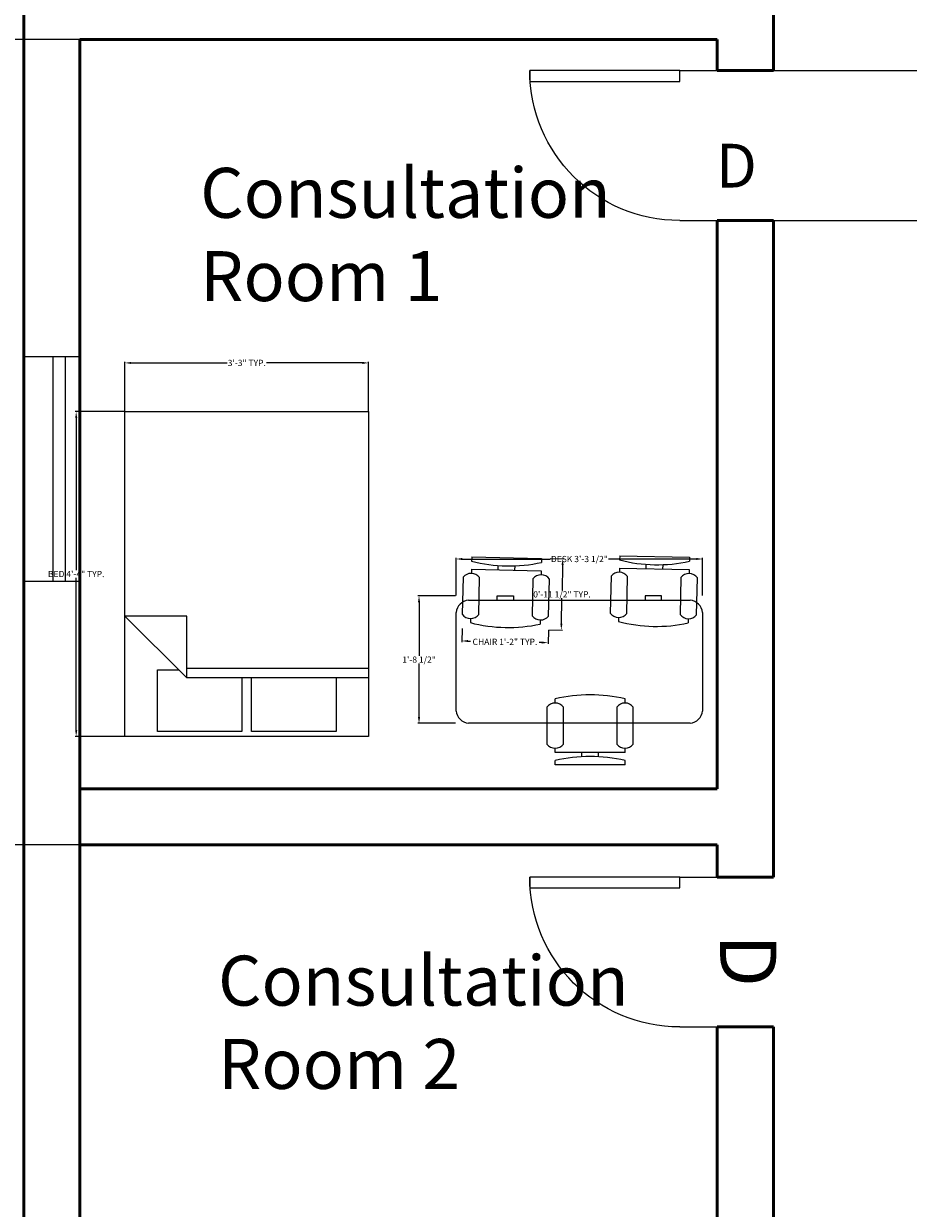
# Model space of a CAD drawing. Units: inches. Extents: x -364 to 705, y -52 to 1250.
# Tile 22 of 34: x 29 to 170, y 648 to 838. Entities that reach past the tile are written whole.
import ezdxf

# ---------------------------------------------------------------- set-up
doc = ezdxf.new("R2010")
doc.units = ezdxf.units.IN
doc.header["$MEASUREMENT"] = 0
for name, color, linetype, lineweight in [('A-ANNO-DIMS', 4, 'Continuous', 18), ('A-ANNO-IDEN', 1, 'Continuous', 18), ('A-AREA-IDEN', 3, 'Continuous', 18), ('A-DOOR', 1, 'Continuous', 25), ('A-FURN', 8, 'Continuous', 18), ('A-GLAZ', 4, 'Continuous', 25), ('A-WALL', 41, 'Continuous', 50)]:
    doc.layers.add(name, color=color, linetype=linetype, lineweight=lineweight)
doc.styles.get("Standard").update_dxf_attribs({"font": 'arial.ttf'})
doc.dimstyles.get("Standard").update_dxf_attribs({"dimtxt": 1, "dimasz": 1, "dimexe": 0.18, "dimexo": 0.0625, "dimgap": 0.09, "dimtad": 0, "dimtih": 1, "dimtoh": 1, "dimdec": 0, "dimzin": 0, "dimdsep": 46, "dimlunit": 3, "dimtxsty": 'Standard', "dimcen": 0.09, "dimadec": 0, "dimazin": 0, "dimtfac": 1, "dimtdec": 0, "dimtofl": 0, "dimtmove": 0, "dimatfit": 3, "dimfxl": 1, "dimtolj": 1, "dimtzin": 0, "dimarcsym": 0})

# ---------------------------------------------------------------- blocks, each defined once
blk = doc.blocks.new('Chair - Desk')
for p, q in [((-8.5, 0), (-8.5, -1)), ((-8.5, 0), (8.5, 0)), ((8.5, 0), (8.5, -1)), ((-2, -3), (-2, -1.9355)), ((2, -1.9576), (2, -3)), ((-10.5, -5), (-10.5, -14)), ((-8.5, -3), (-8.5, -4)), ((-8.5, -3), (8.5, -3)), ((-6.5, -14), (-6.5, -5)), ((6.5, -5), (6.5, -14)), ((8.5, -3), (8.5, -4)), ((10.5, -14), (10.5, -5)), ((-8.5, -15), (-8.5, -16)), ((8.5, -15), (8.5, -16))]:
    blk.add_line(p, q)
for centre, radius, start, end in [((0, 34.625), 36.625, 256.5803, 283.4197), ((-8.5, -6.5), 2.5, 36.8699, 143.1301), ((8.5, -6.5), 2.5, 36.8699, 143.1301), ((-8.5, -12.5), 2.5, 216.8699, 323.1301), ((8.5, -12.5), 2.5, 216.8699, 323.1301), ((0, 19.625), 36.625, 256.5803, 283.4197)]:
    blk.add_arc(centre, radius, start, end)
blk = doc.blocks.new('Desk - 30 x 60 in.')
for p, q in [((-26.999995, 0), (26.999995, 0)), ((-29.999995, -27), (-29.999995, -3)), ((29.999995, -3), (29.999995, -27)), ((26.999995, -30), (-26.999995, -30)), ((-20.000005, -30), (-20.000005, -31)), ((-20.000005, -31), (-16.000005, -31)), ((-16.000005, -31), (-16.000005, -30)), ((15.999995, -31), (15.999995, -30)), ((19.999995, -31), (15.999995, -31)), ((19.999995, -30), (19.999995, -31))]:
    blk.add_line(p, q)
for centre, start, end in [((-26.499995, -3.5), 98.1301, 171.8699), ((26.499995, -3.5), 8.130102, 81.8699), ((-26.499995, -26.5), 188.1301, 261.8699), ((26.499995, -26.5), 278.1301, 351.8699)]:
    blk.add_arc(centre, 3.535534, start, end)
blk = doc.blocks.new('Bed - Queen')
for p, q in [((0, -80.00003), (0, 0)), ((0, 0), (59.99999, 0)), ((59.99999, 0), (59.99999, -80.00003)), ((7.99999, -1.2), (28.79998, -1.2)), ((7.99999, -14.4), (7.99999, -1.2)), ((28.79998, -1.2), (28.79998, -14.4)), ((31.19999, -1.2), (51.99999, -1.2)), ((31.19999, -14.4), (31.19999, -1.2)), ((51.99999, -1.2), (51.99999, -16.4)), ((0, -14.4), (44.8, -14.4)), ((59.99999, -29.6), (44.8, -14.4)), ((44.8, -14.4), (44.8, -29.6)), ((44.8, -16.8), (0, -16.8)), ((51.99999, -16.4), (46.79936, -16.4)), ((44.8, -29.6), (59.99999, -29.6)), ((59.99999, -80.00003), (0, -80.00003))]:
    blk.add_line(p, q)
blk = doc.blocks.new('*U16')
for p, q in [((-24, 0), (-24, 6)), ((0, 0), (0, 6))]:
    blk.add_line(p, q)
blk.add_lwpolyline([(0, 0), (0, -24), (-1.75, -24), (-1.75, 0)], close=True)
blk.add_arc((0, 0), 24, 180, 270)
blk = doc.blocks.new('*D19')
at = {"layer": 'A-ANNO-DIMS', "color": 0, "lineweight": -2, "transparency": 16777216}
for p, q in [((28.52, 986.11), (-248.33, 986.11)), ((-248.15, 985.11), (-248.15, 574.22)), ((-248.15, 149.87), (-248.15, 560.77)), ((28.52, 148.87), (-248.33, 148.87))]:
    blk.add_line(p, q, dxfattribs=at)
at = {"layer": 'A-ANNO-DIMS', "color": 0, "transparency": 16777216}
for points in [[(-248.32, 985.11), (-247.99, 985.11), (-248.15, 986.11)], [(-248.32, 149.87), (-247.99, 149.87), (-248.15, 148.87)]]:
    blk.add_solid(points, dxfattribs=at)
at = {"layer": 'Defpoints', "color": 0, "transparency": 16777216}
for p in [(28.58, 986.11), (-248.15, 148.87), (28.58, 148.87)]:
    blk.add_point(p, dxfattribs=at)
at = {"layer": 'A-ANNO-DIMS', "color": 0, "transparency": 16777216, "insert": (-248.15, 567.49), "char_height": 1, "attachment_point": 5}
blk.add_mtext('\\A1;{\\H13x;69\'-9"}', dxfattribs=at)
blk = doc.blocks.new('*D20')
at = {"layer": 'A-ANNO-DIMS', "color": 0, "lineweight": -2, "transparency": 16777216}
for p, q in [((28.52, 986.11), (-188.21, 986.11)), ((-188.03, 985.11), (-188.03, 917.23)), ((-188.03, 836.11), (-188.03, 904)), ((37.52, 835.11), (-188.21, 835.11))]:
    blk.add_line(p, q, dxfattribs=at)
at = {"layer": 'A-ANNO-DIMS', "color": 0, "transparency": 16777216}
for points in [[(-188.19, 985.11), (-187.86, 985.11), (-188.03, 986.11)], [(-188.19, 836.11), (-187.86, 836.11), (-188.03, 835.11)]]:
    blk.add_solid(points, dxfattribs=at)
at = {"layer": 'Defpoints', "color": 0, "transparency": 16777216}
for p in [(28.58, 986.11), (-188.03, 835.11), (37.58, 835.11)]:
    blk.add_point(p, dxfattribs=at)
at = {"layer": 'A-ANNO-DIMS', "color": 0, "transparency": 16777216, "insert": (-188.03, 910.61), "char_height": 1, "attachment_point": 5}
blk.add_mtext('\\A1;{\\H13x;12\'-7"}', dxfattribs=at)
blk = doc.blocks.new('*D21')
at = {"layer": 'A-ANNO-DIMS', "color": 0, "lineweight": -2, "transparency": 16777216}
for p, q in [((37.52, 835.11), (-188.94, 835.11)), ((-188.76, 834.11), (-188.76, 777.34)), ((-188.76, 707.11), (-188.76, 763.89)), ((37.52, 706.11), (-188.94, 706.11))]:
    blk.add_line(p, q, dxfattribs=at)
at = {"layer": 'A-ANNO-DIMS', "color": 0, "transparency": 16777216}
for points in [[(-188.93, 834.11), (-188.59, 834.11), (-188.76, 835.11)], [(-188.93, 707.11), (-188.59, 707.11), (-188.76, 706.11)]]:
    blk.add_solid(points, dxfattribs=at)
at = {"layer": 'Defpoints', "color": 0, "transparency": 16777216}
for p in [(37.58, 835.11), (-188.76, 706.11), (37.58, 706.11)]:
    blk.add_point(p, dxfattribs=at)
at = {"layer": 'A-ANNO-DIMS', "color": 0, "transparency": 16777216, "insert": (-188.76, 770.61), "char_height": 1, "attachment_point": 5}
blk.add_mtext('\\A1;{\\H13x;10\'-9"}', dxfattribs=at)
blk = doc.blocks.new('*D31')
at = {"layer": 'A-ANNO-DIMS', "color": 0, "lineweight": -2, "transparency": 16777216}
for p, q in [((37.52, 706.11), (-205.07, 706.11)), ((-204.89, 705.11), (-204.89, 648.34)), ((-204.89, 578.11), (-204.89, 634.89)), ((37.52, 577.11), (-205.07, 577.11))]:
    blk.add_line(p, q, dxfattribs=at)
at = {"layer": 'A-ANNO-DIMS', "color": 0, "transparency": 16777216}
for points in [[(-205.06, 705.11), (-204.73, 705.11), (-204.89, 706.11)], [(-205.06, 578.11), (-204.73, 578.11), (-204.89, 577.11)]]:
    blk.add_solid(points, dxfattribs=at)
at = {"layer": 'Defpoints', "color": 0, "transparency": 16777216}
for p in [(37.58, 706.11), (-204.89, 577.11), (37.58, 577.11)]:
    blk.add_point(p, dxfattribs=at)
at = {"layer": 'A-ANNO-DIMS', "color": 0, "transparency": 16777216, "insert": (-204.89, 641.61), "char_height": 1, "attachment_point": 5}
blk.add_mtext('\\A1;{\\H13x;10\'-9"}', dxfattribs=at)
blk = doc.blocks.new('*D40')
at = {"layer": 'A-ANNO-DIMS', "color": 0, "lineweight": -2, "transparency": 16777216}
for p, q in [((98.74, 740.79), (98.7, 738.6)), ((112.56, 740.51), (112.51, 738.33)), ((99.7, 738.76), (100.11, 738.76)), ((111.52, 738.53), (111.11, 738.53))]:
    blk.add_line(p, q, dxfattribs=at)
at = {"layer": 'A-ANNO-DIMS', "color": 0, "transparency": 16777216}
for points in [[(99.71, 738.93), (99.7, 738.6), (98.7, 738.78)], [(111.52, 738.69), (111.51, 738.36), (112.52, 738.51)]]:
    blk.add_solid(points, dxfattribs=at)
at = {"layer": 'Defpoints', "color": 0, "transparency": 16777216}
for p in [(98.75, 740.86), (112.56, 740.58), (112.52, 738.51)]:
    blk.add_point(p, dxfattribs=at)
at = {"layer": 'A-ANNO-DIMS', "color": 0, "transparency": 16777216, "insert": (105.61, 738.64), "char_height": 1, "attachment_point": 5}
blk.add_mtext('\\A1;CHAIR 1\'-2" TYP.', dxfattribs=at)
blk = doc.blocks.new('*D41')
at = {"layer": 'A-ANNO-DIMS', "color": 0, "lineweight": -2, "transparency": 16777216}
for p, q in [((112.85, 751.98), (115.04, 751.93)), ((114.84, 750.94), (114.76, 746.84)), ((114.65, 741.53), (114.73, 745.63)), ((112.62, 740.58), (114.81, 740.53))]:
    blk.add_line(p, q, dxfattribs=at)
at = {"layer": 'A-ANNO-DIMS', "color": 0, "transparency": 16777216}
for points in [[(114.67, 750.94), (115.01, 750.93), (114.86, 751.94)], [(114.48, 741.54), (114.82, 741.53), (114.63, 740.53)]]:
    blk.add_solid(points, dxfattribs=at)
at = {"layer": 'Defpoints', "color": 0, "transparency": 16777216}
for p in [(112.79, 751.98), (114.86, 751.94), (112.56, 740.58)]:
    blk.add_point(p, dxfattribs=at)
at = {"layer": 'A-ANNO-DIMS', "color": 0, "transparency": 16777216, "insert": (114.75, 746.24), "char_height": 1, "attachment_point": 5}
blk.add_mtext('\\A1;0\'-11 1/2" TYP.', dxfattribs=at)
blk = doc.blocks.new('*D52')
at = {"layer": 'A-ANNO-DIMS', "color": 0, "lineweight": -2, "transparency": 16777216}
for p, q in [((97.78, 746.05), (97.78, 752.08)), ((98.78, 751.9), (112.86, 751.9)), ((136.25, 751.9), (122.17, 751.9)), ((137.25, 746.05), (137.25, 752.08))]:
    blk.add_line(p, q, dxfattribs=at)
at = {"layer": 'A-ANNO-DIMS', "color": 0, "transparency": 16777216}
for points in [[(98.78, 752.07), (98.78, 751.74), (97.78, 751.9)], [(136.25, 752.07), (136.25, 751.74), (137.25, 751.9)]]:
    blk.add_solid(points, dxfattribs=at)
at = {"layer": 'Defpoints', "color": 0, "transparency": 16777216}
for p in [(97.78, 751.9), (97.78, 745.98), (137.25, 745.98)]:
    blk.add_point(p, dxfattribs=at)
at = {"layer": 'A-ANNO-DIMS', "color": 0, "transparency": 16777216, "insert": (117.52, 751.9), "char_height": 1, "attachment_point": 5}
blk.add_mtext('\\A1;DESK 3\'-3 1/2"', dxfattribs=at)
blk = doc.blocks.new('*D53')
at = {"layer": 'A-ANNO-DIMS', "color": 0, "lineweight": -2, "transparency": 16777216}
for p, q in [((97.72, 745.98), (91.68, 745.98)), ((91.86, 744.98), (91.86, 736.39)), ((91.86, 726.59), (91.86, 735.18)), ((97.72, 725.59), (91.68, 725.59))]:
    blk.add_line(p, q, dxfattribs=at)
at = {"layer": 'A-ANNO-DIMS', "color": 0, "transparency": 16777216}
for points in [[(91.69, 744.98), (92.03, 744.98), (91.86, 745.98)], [(91.69, 726.59), (92.03, 726.59), (91.86, 725.59)]]:
    blk.add_solid(points, dxfattribs=at)
at = {"layer": 'Defpoints', "color": 0, "transparency": 16777216}
for p in [(97.78, 745.98), (91.86, 725.59), (97.78, 725.59)]:
    blk.add_point(p, dxfattribs=at)
at = {"layer": 'A-ANNO-DIMS', "color": 0, "transparency": 16777216, "insert": (91.86, 735.79), "char_height": 1, "attachment_point": 5}
blk.add_mtext('\\A1;1\'-8 1/2"', dxfattribs=at)
blk = doc.blocks.new('*D64')
at = {"layer": 'A-ANNO-DIMS', "color": 0, "lineweight": -2, "transparency": 16777216}
for p, q in [((44.72, 775.5), (36.8, 775.5)), ((36.98, 774.5), (36.98, 750.09)), ((36.98, 724.5), (36.98, 748.91)), ((44.72, 723.5), (36.8, 723.5))]:
    blk.add_line(p, q, dxfattribs=at)
at = {"layer": 'A-ANNO-DIMS', "color": 0, "transparency": 16777216}
for points in [[(36.82, 774.5), (37.15, 774.5), (36.98, 775.5)], [(36.82, 724.5), (37.15, 724.5), (36.98, 723.5)]]:
    blk.add_solid(points, dxfattribs=at)
at = {"layer": 'Defpoints', "color": 0, "transparency": 16777216}
for p in [(44.78, 775.5), (36.98, 723.5), (44.78, 723.5)]:
    blk.add_point(p, dxfattribs=at)
at = {"layer": 'A-ANNO-DIMS', "color": 0, "transparency": 16777216, "insert": (36.98, 749.5), "char_height": 1, "attachment_point": 5}
blk.add_mtext('\\A1;BED 4\'-4" TYP.', dxfattribs=at)
blk = doc.blocks.new('*D65')
at = {"layer": 'A-ANNO-DIMS', "color": 0, "lineweight": -2, "transparency": 16777216}
for p, q in [((44.78, 775.56), (44.78, 783.48)), ((83.79, 775.56), (83.79, 783.48)), ((45.78, 783.3), (61.15, 783.3)), ((82.79, 783.3), (67.42, 783.3))]:
    blk.add_line(p, q, dxfattribs=at)
at = {"layer": 'A-ANNO-DIMS', "color": 0, "transparency": 16777216}
for points in [[(45.78, 783.46), (45.78, 783.13), (44.78, 783.3)], [(82.79, 783.46), (82.79, 783.13), (83.79, 783.3)]]:
    blk.add_solid(points, dxfattribs=at)
at = {"layer": 'Defpoints', "color": 0, "transparency": 16777216}
for p in [(44.78, 783.3), (44.78, 775.5), (83.79, 775.5)]:
    blk.add_point(p, dxfattribs=at)
at = {"layer": 'A-ANNO-DIMS', "color": 0, "transparency": 16777216, "insert": (64.29, 783.3), "char_height": 1, "attachment_point": 5}
blk.add_mtext('\\A1;3\'-3" TYP.', dxfattribs=at)
blk = doc.blocks.new('*D105')
at = {"layer": 'A-ANNO-DIMS', "color": 0, "lineweight": -2, "transparency": 16777216}
for p, q in [((148.64, 830.11), (703.01, 830.11)), ((702.83, 829.11), (702.83, 818.72)), ((702.83, 807.11), (702.83, 817.51)), ((148.64, 806.11), (703.01, 806.11))]:
    blk.add_line(p, q, dxfattribs=at)
at = {"layer": 'A-ANNO-DIMS', "color": 0, "transparency": 16777216}
for points in [[(702.66, 829.11), (703, 829.11), (702.83, 830.11)], [(702.66, 807.11), (703, 807.11), (702.83, 806.11)]]:
    blk.add_solid(points, dxfattribs=at)
at = {"layer": 'Defpoints', "color": 0, "transparency": 16777216}
for p in [(148.58, 830.11), (148.58, 806.11), (702.83, 806.11)]:
    blk.add_point(p, dxfattribs=at)
at = {"layer": 'A-ANNO-DIMS', "color": 0, "transparency": 16777216, "insert": (702.83, 818.11), "char_height": 1, "attachment_point": 5}
blk.add_mtext('\\A1;2\'-0"', dxfattribs=at)

msp = doc.modelspace()

# ---------------------------------------------------------------- linework, layer by layer
at = {"layer": 'A-GLAZ'}
for p, q in [((33.23, 784.3), (33.23, 748.3)), ((35.23, 784.3), (35.23, 748.3))]:
    msp.add_line(p, q, dxfattribs=at)
msp.add_lwpolyline([(37.58, 784.3), (37.58, 748.3), (28.58, 748.3), (28.58, 784.3)], close=True, dxfattribs=at)
at = {"layer": 'A-WALL'}
for p, q in [((28.58, 11.11), (28.58, 986.11)), ((148.58, 830.11), (148.58, 845.11)), ((139.58, 835.11), (37.58, 835.11)), ((37.58, 586.11), (37.58, 835.11)), ((139.58, 830.11), (139.58, 835.11)), ((139.58, 830.11), (148.58, 830.11)), ((139.58, 806.11), (148.58, 806.11)), ((139.58, 715.11), (139.58, 806.11)), ((148.58, 700.98), (148.58, 806.11)), ((139.58, 715.11), (37.58, 715.11)), ((139.58, 706.11), (37.58, 706.11)), ((139.58, 700.98), (139.58, 706.11)), ((139.58, 700.98), (139.58, 705.98)), ((139.58, 700.98), (148.58, 700.98)), ((139.58, 676.98), (148.58, 676.98)), ((139.58, 586.11), (139.58, 676.98)), ((148.58, 571.14), (148.58, 676.98))]:
    msp.add_line(p, q, dxfattribs=at)

# ---------------------------------------------------------------- block references
at = {"layer": 'A-DOOR', "xscale": -1, "rotation": 270.0000000000011}
for p in [(133.58, 830.11), (133.58, 700.98)]:
    msp.add_blockref('*U16', p, dxfattribs=at)
at = {"layer": 'A-FURN'}
for name, p, xscale, yscale, zscale, rotation in [('Bed - Queen', (83.79, 723.5), 0.6500148169160638, 0.6500148169160638, 0.6500148169160638, 180), ('Chair - Desk', (105.88, 752.12), 0.6578509577389904, 0.6578509577389904, 0.6578509577389904, 358.8399543093713), ('Chair - Desk', (129.57, 752.3), 0.6578509577389904, 0.6578509577389904, 0.6578509577389904, 358.8399543093713), ('Desk - 30 x 60 in.', (117.52, 725.59), 0.6578509577389904, 0.6578509577389904, 0.6578509577389904, 180), ('Chair - Desk', (119.24, 718.97), 0.6578509577389904, 0.6578509577389904, 0.6578509577389904, 180)]:
    msp.add_blockref(name, p, dxfattribs=dict(at, xscale=xscale, yscale=yscale, zscale=zscale, rotation=rotation))

# ---------------------------------------------------------------- texts
at = {"layer": 'A-ANNO-IDEN', "insert": (139.37, 811.38), "char_height": 7, "attachment_point": 7}
msp.add_mtext_dynamic_manual_height_columns('D', width=150.7943, gutter_width=1, heights=[0], dxfattribs=at)
at = {"layer": 'A-ANNO-IDEN', "insert": (149.06, 691.82), "char_height": 9, "attachment_point": 1, "rotation": 270}
msp.add_mtext_dynamic_manual_height_columns('D', width=16.916, gutter_width=1, heights=[0], dxfattribs=at)
at = {"layer": 'A-AREA-IDEN', "char_height": 8, "attachment_point": 1}
for s, width, insert in [('Consultation Room 1', 91.7461, (56.83, 814.53)), ('Consultation Room 2', 84.2125, (59.69, 688.39))]:
    msp.add_mtext_dynamic_manual_height_columns(s, width=width, gutter_width=1, heights=[0], dxfattribs=dict(at, insert=insert))

# ---------------------------------------------------------------- dimensions: what is measured, and where the dimension line sits
at = {"layer": 'A-ANNO-DIMS'}
for base, p1, p2, angle, text, override, picture, middle in [((-248.15, 148.87), (28.58, 986.11), (28.58, 148.87), 90, '{\\H13x;<>}', {"dimclrd": 0, "dimclre": 0, "dimclrt": 0}, '*D19', (-248.15, 567.49)), ((-188.76, 706.11), (37.58, 835.11), (37.58, 706.11), 90, '{\\H13x;<>}', {"dimclrd": 0, "dimclre": 0, "dimclrt": 0}, '*D21', (-188.76, 770.61)), ((44.78, 783.3), (83.79, 775.5), (44.78, 775.5), 180, '<> TYP.', {"dimdec": 1, "dimlfac": 1, "dimrnd": 0, "dimzin": 1, "dimdsep": 46, "dimlunit": 4, "dimfrac": 2}, '*D65', (64.29, 783.3)), ((36.98, 723.5), (44.78, 775.5), (44.78, 723.5), 270, 'BED <> TYP.', {"dimdec": 1, "dimlfac": 1, "dimrnd": 0, "dimzin": 1, "dimdsep": 46, "dimlunit": 4, "dimfrac": 2}, '*D64', (36.98, 749.5)), ((97.78, 751.9), (137.25, 745.98), (97.78, 745.98), 180, 'DESK <>', {"dimdec": 1, "dimlfac": 1, "dimrnd": 0, "dimzin": 1, "dimdsep": 46, "dimlunit": 4, "dimfrac": 2}, '*D52', (117.52, 751.9)), ((114.86, 751.94), (112.56, 740.58), (112.79, 751.98), 88.84, '<> TYP.', {"dimdec": 1, "dimlfac": 1, "dimrnd": 0, "dimzin": 1, "dimdsep": 46, "dimlunit": 4, "dimfrac": 2}, '*D41', (114.75, 746.24)), ((112.52, 738.51), (98.75, 740.86), (112.56, 740.58), 358.84, 'CHAIR <> TYP.', {"dimdec": 1, "dimlfac": 1, "dimrnd": 0, "dimzin": 1, "dimdsep": 46, "dimlunit": 4, "dimfrac": 2}, '*D40', (105.61, 738.64)), ((-204.89, 577.11), (37.58, 706.11), (37.58, 577.11), 90, '{\\H13x;<>}', {"dimclrd": 0, "dimclre": 0, "dimclrt": 0}, '*D31', (-204.89, 641.61))]:
    dim = msp.add_linear_dim(base=base, p1=p1, p2=p2, angle=angle, text=text, dimstyle='Standard', override=override, dxfattribs=at)
    dim.commit()
    dim.dimension.update_dxf_attribs({"geometry": picture, "text_midpoint": middle})
dim = msp.add_linear_dim(base=(-188.03, 835.11), p1=(28.58, 986.11), p2=(37.58, 835.11), angle=90, text='{\\H13x;<>}', dimstyle='Standard', override={"dimclrd": 0, "dimclre": 0, "dimclrt": 0}, dxfattribs=at)
dim.commit()
dim.dimension.update_dxf_attribs({"geometry": '*D20', "text_midpoint": (-188.03, 910.61), "dimtype": 160})
for base, p1, p2, angle, picture, middle in [((702.83, 806.11), (148.58, 830.11), (148.58, 806.11), 90, '*D105', (702.83, 818.11)), ((91.86, 725.59), (97.78, 745.98), (97.78, 725.59), 270, '*D53', (91.86, 735.79))]:
    dim = msp.add_linear_dim(base=base, p1=p1, p2=p2, angle=angle, dimstyle='Standard', override={"dimdec": 1, "dimlfac": 1, "dimrnd": 0, "dimzin": 1, "dimdsep": 46, "dimlunit": 4, "dimfrac": 2}, dxfattribs=at)
    dim.commit()
    dim.dimension.update_dxf_attribs({"geometry": picture, "text_midpoint": middle})

doc.saveas('drawing.dxf')
